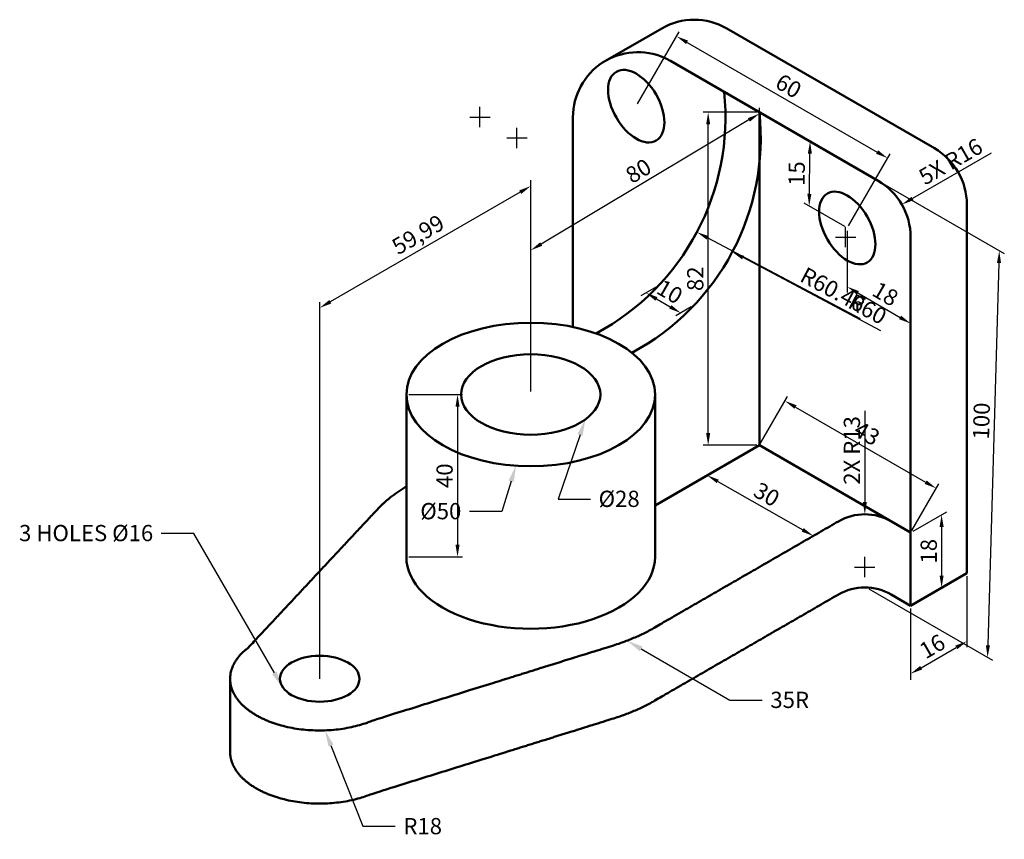
# Model space of a CAD drawing. Units: millimetres. Extents: x -6 to 237, y 25 to 227.
import ezdxf
from ezdxf import colors
from ezdxf.entities.mleader import LeaderData, LeaderLine
from ezdxf.math import Vec2, Vec3

# ---------------------------------------------------------------- set-up
doc = ezdxf.new("R2010")
doc.units = ezdxf.units.MM
doc.layers.add('M-DIMS', color=2, linetype='Continuous', lineweight=25)
doc.layers.add('M-OUTL', color=7, linetype='Continuous', lineweight=50)
doc.styles.get("Standard").update_dxf_attribs({"font": 'arial.ttf'})
doc.dimstyles.new('ISO-25', dxfattribs={"dimtxt": 4, "dimasz": 3, "dimexe": 1.25, "dimexo": 0.625, "dimtad": 1, "dimtxsty": 'Standard', "dimcen": 2.5, "dimadec": 0, "dimazin": 0, "dimtfac": 1, "dimtofl": 0, "dimtmove": 0, "dimatfit": 3, "dimfxl": 1, "dimarcsym": 0})

# ---------------------------------------------------------------- blocks, each defined once
blk = doc.blocks.new('*D1')
at = {"layer": 'Defpoints', "color": 0, "transparency": 16777216}
for p in [(227.4, 90.98), (213.54, 82.98), (227.4, 74.21)]:
    blk.add_point(p, dxfattribs=at)
at = {"layer": 'M-DIMS', "color": 0, "lineweight": -2, "transparency": 16777216}
for p, q in [((227.4, 90.26), (227.4, 72.76)), ((213.54, 82.26), (213.54, 64.76)), ((216.14, 67.71), (224.8, 72.71))]:
    blk.add_line(p, q, dxfattribs=at)
at = {"layer": 'M-DIMS', "color": 0, "transparency": 16777216}
for points in [[(224.55, 73.14), (225.05, 72.27), (227.4, 74.21)], [(215.89, 68.14), (216.39, 67.27), (213.54, 66.21)]]:
    blk.add_solid(points, dxfattribs=at)
at = {"layer": 'M-DIMS', "color": 0, "transparency": 16777216, "insert": (219.14, 72.52), "char_height": 4, "attachment_point": 5, "rotation": 30}
blk.add_mtext('16', dxfattribs=at)
blk = doc.blocks.new('*D2')
at = {"layer": 'Defpoints', "color": 0, "transparency": 16777216}
for p in [(145.99, 205.98), (207.88, 193.18), (197.95, 175.98)]:
    blk.add_point(p, dxfattribs=at)
at = {"layer": 'M-DIMS', "color": 0, "lineweight": -2, "transparency": 16777216}
for p, q in [((146.3, 206.52), (156.55, 224.26)), ((158.52, 221.68), (205.29, 194.68)), ((198.27, 176.52), (208.51, 194.26))]:
    blk.add_line(p, q, dxfattribs=at)
at = {"layer": 'M-DIMS', "color": 0, "transparency": 16777216}
for points in [[(158.77, 222.11), (158.27, 221.25), (155.92, 223.18)], [(205.54, 195.11), (205.04, 194.25), (207.88, 193.18)]]:
    blk.add_solid(points, dxfattribs=at)
at = {"layer": 'M-DIMS', "color": 0, "transparency": 16777216, "insert": (183.24, 210.49), "char_height": 4, "attachment_point": 5, "rotation": 330}
blk.add_mtext('60', dxfattribs=at)
blk = doc.blocks.new('*D3')
at = {"layer": 'Defpoints', "color": 0, "transparency": 16777216}
for p in [(188.78, 197.27), (198.15, 191.87), (197.95, 175.98)]:
    blk.add_point(p, dxfattribs=at)
at = {"layer": 'M-DIMS', "color": 0, "lineweight": -2, "transparency": 16777216}
for p, q in [((197.53, 192.22), (187.54, 197.99)), ((188.62, 184.39), (188.74, 194.27)), ((197.33, 176.34), (187.34, 182.1))]:
    blk.add_line(p, q, dxfattribs=at)
at = {"layer": 'M-DIMS', "color": 0, "transparency": 16777216}
for points in [[(188.24, 194.28), (189.24, 194.27), (188.78, 197.27)], [(188.12, 184.39), (189.12, 184.38), (188.58, 181.39)]]:
    blk.add_solid(points, dxfattribs=at)
at = {"layer": 'M-DIMS', "color": 0, "transparency": 16777216, "insert": (186.01, 189.36), "char_height": 4, "attachment_point": 5, "rotation": 89.2938}
blk.add_mtext('15', dxfattribs=at)
blk = doc.blocks.new('*D4')
at = {"layer": 'Defpoints', "color": 0, "transparency": 16777216}
for p in [(197.95, 175.98), (213.54, 166.92), (213.54, 152.46)]:
    blk.add_point(p, dxfattribs=at)
at = {"layer": 'M-DIMS', "color": 0, "lineweight": -2, "transparency": 16777216}
for p, q in [((197.95, 175.26), (197.95, 160.07)), ((213.54, 166.2), (213.54, 151.01)), ((200.55, 160.01), (210.95, 153.96))]:
    blk.add_line(p, q, dxfattribs=at)
at = {"layer": 'M-DIMS', "color": 0, "transparency": 16777216}
for points in [[(200.8, 160.44), (200.3, 159.57), (197.95, 161.51)], [(211.2, 154.4), (210.7, 153.53), (213.54, 152.46)]]:
    blk.add_solid(points, dxfattribs=at)
at = {"layer": 'M-DIMS', "color": 0, "transparency": 16777216, "insert": (207.09, 159.29), "char_height": 4, "attachment_point": 5, "rotation": 329.8439}
blk.add_mtext('18', dxfattribs=at)
blk = doc.blocks.new('*D5')
at = {"layer": 'Defpoints', "color": 0, "transparency": 16777216}
for p in [(163.47, 115.07), (189.58, 100.16), (189.58, 100.16)]:
    blk.add_point(p, dxfattribs=at)
at = {"layer": 'M-DIMS', "color": 0, "lineweight": -2, "transparency": 16777216}
for p, q in [((164.09, 115.43), (164.72, 115.79)), ((166.07, 113.58), (186.98, 101.64)), ((190.21, 100.52), (190.83, 100.88))]:
    blk.add_line(p, q, dxfattribs=at)
at = {"layer": 'M-DIMS', "color": 0, "transparency": 16777216}
for points in [[(166.32, 114.01), (165.82, 113.15), (163.47, 115.07)], [(187.22, 102.08), (186.73, 101.21), (189.58, 100.16)]]:
    blk.add_solid(points, dxfattribs=at)
at = {"layer": 'M-DIMS', "color": 0, "transparency": 16777216, "insert": (177.85, 109.93), "char_height": 4, "attachment_point": 5, "rotation": 330.2759}
blk.add_mtext('30', dxfattribs=at)
blk = doc.blocks.new('*D6')
at = {"layer": 'Defpoints', "color": 0, "transparency": 16777216}
for p in [(213.54, 100.98), (221.18, 87.39), (213.54, 82.98)]:
    blk.add_point(p, dxfattribs=at)
at = {"layer": 'M-DIMS', "color": 0, "lineweight": -2, "transparency": 16777216}
for p, q in [((214.17, 101.34), (222.43, 106.11)), ((221.18, 102.39), (221.18, 90.39)), ((214.17, 83.34), (222.43, 88.11))]:
    blk.add_line(p, q, dxfattribs=at)
at = {"layer": 'M-DIMS', "color": 0, "transparency": 16777216}
for points in [[(220.68, 102.39), (221.68, 102.39), (221.18, 105.39)], [(220.68, 90.39), (221.68, 90.39), (221.18, 87.39)]]:
    blk.add_solid(points, dxfattribs=at)
at = {"layer": 'M-DIMS', "color": 0, "transparency": 16777216, "insert": (218.52, 96.39), "char_height": 4, "attachment_point": 5, "rotation": 90}
blk.add_mtext('18', dxfattribs=at)
blk = doc.blocks.new('*D7')
at = {"layer": 'Defpoints', "color": 0, "transparency": 16777216}
for p in [(68.05, 156.31), (120.01, 134.98), (68.05, 105)]:
    blk.add_point(p, dxfattribs=at)
at = {"layer": 'M-DIMS', "color": 0, "lineweight": -2, "transparency": 16777216}
for p, q in [((120.01, 135.7), (120.01, 187.73)), ((117.41, 184.79), (70.65, 157.81)), ((68.05, 105.72), (68.05, 157.75))]:
    blk.add_line(p, q, dxfattribs=at)
at = {"layer": 'M-DIMS', "color": 0, "transparency": 16777216}
for points in [[(117.16, 185.22), (117.66, 184.35), (120.01, 186.29)], [(70.4, 158.24), (70.9, 157.38), (68.05, 156.31)]]:
    blk.add_solid(points, dxfattribs=at)
at = {"layer": 'M-DIMS', "color": 0, "transparency": 16777216, "insert": (92.52, 173.92), "char_height": 4, "attachment_point": 5, "rotation": 29.9808}
blk.add_mtext('59,99', dxfattribs=at)
blk = doc.blocks.new('*D8')
at = {"layer": 'Defpoints', "color": 0, "transparency": 16777216}
for p in [(176.3, 203.27), (120.01, 170.48), (120.01, 169.63)]:
    blk.add_point(p, dxfattribs=at)
at = {"layer": 'M-DIMS', "color": 0, "lineweight": -2, "transparency": 16777216}
for p, q in [((176.3, 203.99), (176.3, 205.58)), ((173.73, 202.59), (122.59, 172.02)), ((120.01, 170.35), (120.01, 171.94))]:
    blk.add_line(p, q, dxfattribs=at)
at = {"layer": 'M-DIMS', "color": 0, "transparency": 16777216}
for points in [[(173.47, 203.01), (173.98, 202.16), (176.3, 204.12)], [(122.33, 172.45), (122.84, 171.59), (120.01, 170.48)]]:
    blk.add_solid(points, dxfattribs=at)
at = {"layer": 'M-DIMS', "color": 0, "transparency": 16777216, "insert": (146.79, 189.59), "char_height": 4, "attachment_point": 5, "rotation": 30.8638}
blk.add_mtext('80', dxfattribs=at)
blk = doc.blocks.new('*D9')
at = {"layer": 'Defpoints', "color": 0, "transparency": 16777216}
for p in [(151.56, 161.87), (160.18, 156.89), (156.97, 155.05)]:
    blk.add_point(p, dxfattribs=at)
at = {"layer": 'M-DIMS', "color": 0, "lineweight": -2, "transparency": 16777216}
for p, q in [((150.94, 161.5), (147.11, 159.3)), ((150.96, 158.52), (154.38, 156.55)), ((159.55, 156.53), (155.72, 154.32))]:
    blk.add_line(p, q, dxfattribs=at)
at = {"layer": 'M-DIMS', "color": 0, "transparency": 16777216}
for points in [[(151.21, 158.95), (150.71, 158.08), (148.36, 160.02)], [(154.63, 156.98), (154.13, 156.11), (156.97, 155.05)]]:
    blk.add_solid(points, dxfattribs=at)
at = {"layer": 'M-DIMS', "color": 0, "transparency": 16777216, "insert": (154, 159.84), "char_height": 4, "attachment_point": 5, "rotation": 330}
blk.add_mtext('10', dxfattribs=at)
blk = doc.blocks.new('*D10')
at = {"layer": 'Defpoints', "color": 0, "transparency": 16777216}
for p in [(205.54, 187.6), (202.65, 87.47), (232.49, 70.24)]:
    blk.add_point(p, dxfattribs=at)
at = {"layer": 'M-DIMS', "color": 0, "lineweight": -2, "transparency": 16777216}
for p, q in [((206.16, 187.24), (236.61, 169.66)), ((235.3, 167.37), (232.58, 73.24)), ((203.26, 87.11), (233.72, 69.53))]:
    blk.add_line(p, q, dxfattribs=at)
at = {"layer": 'M-DIMS', "color": 0, "transparency": 16777216}
for points in [[(234.8, 167.38), (235.8, 167.35), (235.38, 170.37)], [(232.08, 73.25), (233.08, 73.22), (232.49, 70.24)]]:
    blk.add_solid(points, dxfattribs=at)
at = {"layer": 'M-DIMS', "color": 0, "transparency": 16777216, "insert": (231.5, 128.44), "char_height": 4, "attachment_point": 5, "rotation": 88.345}
blk.add_mtext('100', dxfattribs=at)
blk = doc.blocks.new('*D11')
at = {"layer": 'Defpoints', "color": 0, "transparency": 16777216}
for p in [(89.39, 134.98), (89.39, 94.98), (101.99, 94.98)]:
    blk.add_point(p, dxfattribs=at)
at = {"layer": 'M-DIMS', "color": 0, "lineweight": -2, "transparency": 16777216}
for p, q in [((90.02, 134.98), (103.24, 134.98)), ((101.99, 131.98), (101.99, 97.98)), ((90.02, 94.98), (103.24, 94.98))]:
    blk.add_line(p, q, dxfattribs=at)
at = {"layer": 'M-DIMS', "color": 0, "transparency": 16777216}
for points in [[(101.49, 131.98), (102.49, 131.98), (101.99, 134.98)], [(101.49, 97.98), (102.49, 97.98), (101.99, 94.98)]]:
    blk.add_solid(points, dxfattribs=at)
at = {"layer": 'M-DIMS', "color": 0, "transparency": 16777216, "insert": (99.32, 114.98), "char_height": 4, "attachment_point": 5, "rotation": 90}
blk.add_mtext('40', dxfattribs=at)
blk = doc.blocks.new('*D12')
at = {"layer": 'Defpoints', "color": 0, "transparency": 16777216}
for p in [(176.3, 122.48), (219.84, 111.89), (213.54, 100.98)]:
    blk.add_point(p, dxfattribs=at)
at = {"layer": 'M-DIMS', "color": 0, "lineweight": -2, "transparency": 16777216}
for p, q in [((176.61, 123.02), (183.23, 134.47)), ((185.2, 131.89), (217.24, 113.39)), ((213.85, 101.52), (220.47, 112.97))]:
    blk.add_line(p, q, dxfattribs=at)
at = {"layer": 'M-DIMS', "color": 0, "transparency": 16777216}
for points in [[(185.45, 132.32), (184.95, 131.46), (182.6, 133.39)], [(217.49, 113.82), (216.99, 112.96), (219.84, 111.89)]]:
    blk.add_solid(points, dxfattribs=at)
at = {"layer": 'M-DIMS', "color": 0, "transparency": 16777216, "insert": (202.56, 124.95), "char_height": 4, "attachment_point": 5, "rotation": 330}
blk.add_mtext('43', dxfattribs=at)
blk = doc.blocks.new('*D13')
at = {"layer": 'Defpoints', "color": 0, "transparency": 16777216}
for p in [(163.7, 204.48), (176.3, 204.48), (176.3, 122.48)]:
    blk.add_point(p, dxfattribs=at)
at = {"layer": 'M-DIMS', "color": 0, "lineweight": -2, "transparency": 16777216}
for p, q in [((175.68, 204.48), (162.45, 204.48)), ((163.7, 125.48), (163.7, 201.48)), ((175.68, 122.48), (162.45, 122.48))]:
    blk.add_line(p, q, dxfattribs=at)
at = {"layer": 'M-DIMS', "color": 0, "transparency": 16777216}
for points in [[(163.2, 201.48), (164.2, 201.48), (163.7, 204.48)], [(163.2, 125.48), (164.2, 125.48), (163.7, 122.48)]]:
    blk.add_solid(points, dxfattribs=at)
at = {"layer": 'M-DIMS', "color": 0, "transparency": 16777216, "insert": (161.04, 163.48), "char_height": 4, "attachment_point": 5, "rotation": 90}
blk.add_mtext('82', dxfattribs=at)
blk = doc.blocks.new('*D14')
at = {"layer": 'Defpoints', "color": 0, "transparency": 16777216}
for p in [(116.63, 198.17), (169.65, 170.08)]:
    blk.add_point(p, dxfattribs=at)
at = {"layer": 'M-DIMS', "color": 0, "lineweight": -2, "transparency": 16777216}
for p, q in [((116.63, 195.67), (116.63, 200.67)), ((114.13, 198.17), (119.13, 198.17)), ((206.23, 150.69), (172.3, 168.67))]:
    blk.add_line(p, q, dxfattribs=at)
at = {"layer": 'M-DIMS', "color": 0, "transparency": 16777216}
blk.add_solid([(172.53, 169.11), (172.07, 168.23), (169.65, 170.08)], dxfattribs=at)
at = {"layer": 'M-DIMS', "color": 0, "transparency": 16777216, "insert": (202.71, 155.58), "char_height": 4, "attachment_point": 5, "rotation": 332.0773}
blk.add_mtext('R60', dxfattribs=at)
blk = doc.blocks.new('*D15')
at = {"layer": 'Defpoints', "color": 0, "transparency": 16777216}
for p in [(107.5, 203.27), (160.92, 174.95)]:
    blk.add_point(p, dxfattribs=at)
at = {"layer": 'M-DIMS', "color": 0, "lineweight": -2, "transparency": 16777216}
for p, q in [((107.5, 200.77), (107.5, 205.77)), ((105, 203.27), (110, 203.27)), ((201.18, 153.62), (163.57, 173.55))]:
    blk.add_line(p, q, dxfattribs=at)
at = {"layer": 'M-DIMS', "color": 0, "transparency": 16777216}
blk.add_solid([(163.81, 173.99), (163.34, 173.11), (160.92, 174.95)], dxfattribs=at)
at = {"layer": 'M-DIMS', "color": 0, "transparency": 16777216, "insert": (194.23, 160.32), "char_height": 4, "attachment_point": 5, "rotation": 332.0776}
blk.add_mtext('R60.46', dxfattribs=at)
blk = doc.blocks.new('*D16')
at = {"layer": 'Defpoints', "color": 0, "transparency": 16777216}
for p in [(211.4, 181.74), (197.54, 173.74)]:
    blk.add_point(p, dxfattribs=at)
at = {"layer": 'M-DIMS', "color": 0, "lineweight": -2, "transparency": 16777216}
for p, q in [((233.4, 194.44), (214, 183.24)), ((197.54, 171.24), (197.54, 176.24)), ((195.04, 173.74), (200.04, 173.74))]:
    blk.add_line(p, q, dxfattribs=at)
at = {"layer": 'M-DIMS', "color": 0, "transparency": 16777216}
blk.add_solid([(213.75, 183.67), (214.25, 182.81), (211.4, 181.74)], dxfattribs=at)
at = {"layer": 'M-DIMS', "color": 0, "transparency": 16777216, "insert": (223.66, 191.9), "char_height": 4, "attachment_point": 5, "rotation": 29.9982}
blk.add_mtext('5X R16', dxfattribs=at)
blk = doc.blocks.new('*D17')
at = {"layer": 'Defpoints', "color": 0, "transparency": 16777216}
for p in [(202.27, 105.47), (202.27, 92.47)]:
    blk.add_point(p, dxfattribs=at)
at = {"layer": 'M-DIMS', "color": 0, "lineweight": -2, "transparency": 16777216}
for p, q in [((202.27, 130.94), (202.27, 108.47)), ((202.27, 89.97), (202.27, 94.97)), ((199.77, 92.47), (204.77, 92.47))]:
    blk.add_line(p, q, dxfattribs=at)
at = {"layer": 'M-DIMS', "color": 0, "transparency": 16777216}
blk.add_solid([(201.77, 108.47), (202.77, 108.47), (202.27, 105.47)], dxfattribs=at)
at = {"layer": 'M-DIMS', "color": 0, "transparency": 16777216, "insert": (199.6, 121.21), "char_height": 4, "attachment_point": 5, "rotation": 89.9994}
blk.add_mtext('2X R13', dxfattribs=at)

msp = doc.modelspace()

# ---------------------------------------------------------------- linework, layer by layer
at = {"layer": 'M-DIMS'}
msp.add_line((68.049, 64.978), (68.049, 107.557), dxfattribs=at)
at = {"layer": 'M-OUTL'}
for p, q in [((138.403, 217.122), (152.259, 225.122)), ((219.398, 195.597), (168.259, 225.122)), ((205.541, 187.597), (154.403, 217.122)), ((205.541, 187.597), (154.403, 217.122)), ((176.302, 204.478), (176.302, 122.478)), ((130.403, 203.265), (130.403, 151.606)), ((227.398, 90.978), (227.398, 181.74)), ((213.541, 82.978), (213.541, 173.74)), ((89.392, 134.978), (89.392, 94.978)), ((150.629, 134.978), (150.629, 94.978)), ((176.302, 122.478), (150.629, 107.656)), ((213.541, 100.978), (176.302, 122.478)), ((213.541, 82.978), (213.541, 100.978)), ((213.541, 82.978), (227.398, 90.978)), ((208.773, 85.731), (213.541, 82.978)), ((46.004, 46.922), (46.004, 64.978))]:
    msp.add_line(p, q, dxfattribs=at)
for centre, radius, start, end in [((160.259, 211.265), 16, 60, 120), ((146.403, 203.265), 16, 65.96309, 180), ((146.403, 203.265), 16, 60, 65.96309), ((107.498, 203.267), 60.464, 298.25907, 5.89628), ((116.634, 198.175), 60, 298.12497, 6.03038), ((211.398, 181.74), 16, 0, 60), ((197.541, 173.74), 16, 0, 60), ((202.273, 92.473), 13, 60, 120), ((202.273, 74.473), 13, 60, 120)]:
    msp.add_arc(centre, radius, start, end, dxfattribs=at)
for centre, major_axis in [((145.991, 205.978), (4.899, -8.485)), ((197.953, 175.978), (4.899, -8.485)), ((120.011, 134.978), (-30.619, 0)), ((120.011, 134.978), (-17.146, 0)), ((68.049, 64.978), (-9.798, 0))]:
    msp.add_ellipse(centre, major_axis=major_axis, ratio=0.5773503, dxfattribs=at)
msp.add_ellipse((120.011, 94.978), major_axis=(-30.619, 0), ratio=0.5773503, start_param=0, end_param=3.1415927, dxfattribs=at)
for points, weights, knots in [([(89.392, 112.299), (84.799, 109.592), (81.819, 106.216), (66.16, 89.449), (50.501, 72.682), (39.014, 63.961), (52.243, 56.105), (65.472, 48.25), (80.895, 54.634), (110.426, 63.853), (139.957, 73.072), (146.223, 74.974), (151.097, 77.938), (173.435, 90.834), (195.773, 103.731)], [0.996613645118, 0.986806868253, 1, 1, 1, 0.757877776403, 1, 0.757877776403, 1, 1, 1, 0.98663647273, 1, 1, 1], [1.0447145, 1.0447145, 1.0447145, 1.3484128, 1.3484128, 2.3484128, 2.3484128, 3.7698975, 3.7698975, 5.1913822, 5.1913822, 6.1913822, 6.1913822, 6.5187157, 6.5187157, 7.3917018, 7.3917018, 7.3917018]), ([(46.004, 46.922), (46.043, 41.787), (52.243, 38.105), (65.472, 30.25), (80.895, 36.634), (110.426, 45.853), (139.957, 55.072), (146.223, 56.974), (151.097, 59.938), (173.435, 72.834), (195.773, 85.731)], [0.879633594104, 0.86976818109, 1, 0.757877776403, 1, 1, 1, 0.98663647273, 1, 1, 1], [3.0053145, 3.0053145, 3.0053145, 3.7698975, 3.7698975, 5.1913822, 5.1913822, 6.1913822, 6.1913822, 6.5187157, 6.5187157, 7.3917018, 7.3917018, 7.3917018])]:
    msp.add_rational_spline(points, weights, degree=2, knots=knots, dxfattribs=at)

# ---------------------------------------------------------------- dimensions: what is measured, and where the dimension line sits
at = {"layer": 'M-DIMS'}
for p1, p2, distance, picture, middle in [((145.991, 205.978), (197.953, 175.978), 19.862, '*D2', (183.237, 210.489)), ((120.011, 134.978), (68.049, 105.001), -44.443, '*D7', (92.516, 173.921)), ((213.541, 100.978), (213.541, 82.978), 7.642, '*D6', (218.516, 96.39)), ((213.541, 82.978), (227.398, 90.978), -14.523, '*D1', (219.136, 72.518))]:
    dim = msp.add_aligned_dim(p1=p1, p2=p2, distance=distance, dimstyle='ISO-25', override={"dimclrd": 0, "dimclre": 0, "dimclrt": 0}, dxfattribs=at)
    dim.commit()
    dim.dimension.update_dxf_attribs({"geometry": picture, "text_midpoint": middle})
for center, mpoint, override, picture, middle in [((107.498, 203.267), (160.923, 174.953), {"dimdec": 2, "dimlfac": 1, "dimrnd": 0, "dimzin": 0, "dimdsep": 46, "dimlunit": 2}, '*D15', (192.978, 157.965)), ((116.634, 198.175), (169.649, 170.078), {"dimdec": 0, "dimlfac": 1, "dimrnd": 0, "dimzin": 0, "dimdsep": 46, "dimlunit": 2}, '*D14', (201.458, 153.22))]:
    dim = msp.add_radius_dim(center=center, mpoint=mpoint, dimstyle='ISO-25', override=override, dxfattribs=at)
    dim.commit()
    dim.dimension.update_dxf_attribs({"geometry": picture, "text_midpoint": middle, "dimtype": 164})
for p1, p2, distance, text, picture, middle in [((176.302, 203.267), (120.011, 169.625), -0.736, '80', '*D8', (146.788, 189.593)), ((197.953, 175.978), (198.149, 191.865), 9.435, '15', '*D3', (186.015, 189.364)), ((197.953, 175.978), (213.541, 166.921), -12.507, '18', '*D4', (207.087, 159.291)), ((151.564, 161.866), (160.176, 156.894), -3.202, '10', '*D9', (154.002, 159.841)), ((163.466, 115.067), (189.581, 100.156), 0, '30', '*D5', (177.847, 109.929))]:
    dim = msp.add_aligned_dim(p1=p1, p2=p2, distance=distance, text=text, dimstyle='ISO-25', override={"dimclrd": 0, "dimclre": 0, "dimclrt": 0}, dxfattribs=at)
    dim.commit()
    dim.dimension.update_dxf_attribs({"geometry": picture, "text_midpoint": middle})
for base, p1, p2, angle, picture, middle in [((163.702, 204.478), (176.302, 122.478), (176.302, 204.478), 90, '*D13', (161.035, 163.478)), ((101.992, 94.978), (89.392, 134.978), (89.392, 94.978), 270, '*D11', (99.325, 114.978)), ((219.841, 111.89), (176.302, 122.478), (213.541, 100.978), 330, '*D12', (202.556, 124.951))]:
    dim = msp.add_linear_dim(base=base, p1=p1, p2=p2, angle=angle, dimstyle='ISO-25', override={"dimdec": 0, "dimlfac": 1, "dimrnd": 0, "dimzin": 0, "dimdsep": 46, "dimlunit": 2}, dxfattribs=at)
    dim.commit()
    dim.dimension.update_dxf_attribs({"geometry": picture, "text_midpoint": middle})
for center, mpoint, text, picture, middle in [((197.541, 173.74), (211.398, 181.74), '5X <>', '*D16', (223.661, 191.9)), ((202.273, 92.473), (202.273, 105.473), '2X <>', '*D17', (199.605, 121.208))]:
    dim = msp.add_radius_dim(center=center, mpoint=mpoint, text=text, dimstyle='ISO-25', override={"dimdec": 0, "dimlfac": 1, "dimrnd": 0, "dimzin": 0, "dimdsep": 46, "dimlunit": 2}, dxfattribs=at)
    dim.commit()
    dim.dimension.update_dxf_attribs({"geometry": picture, "text_midpoint": middle})
dim = msp.add_linear_dim(base=(232.491, 70.238), p1=(205.541, 187.597), p2=(202.648, 87.467), angle=268.345, text='100', dimstyle='ISO-25', override={"dimclrd": 0, "dimclre": 0, "dimclrt": 0}, dxfattribs=at)
dim.commit()
dim.dimension.update_dxf_attribs({"geometry": '*D10', "text_midpoint": (234.17, 128.359), "dimtype": 161})

# ---------------------------------------------------------------- leaders
ml = msp.add_multileader_mtext('Standard', dxfattribs=at)
ml.set_content('%%C28', color=256)
ml.set_leader_properties()
ml.build(insert=Vec2(0, 0))
ctx = ml.context
ctx.base_point, ctx.plane_origin = Vec3(134.731, 109.208), Vec3(133.453, 128.832)
notes = []
notes.append((ctx, [(0, (1, 1, 0), (126.731, 109.208), (1, 0), 8, [(0, [(133.453, 128.832)], 0, [])])]))
ctx.mtext.insert, ctx.mtext.flow_direction = Vec3(136.731, 111.288), 5
ml = msp.add_multileader_mtext('Standard', dxfattribs=at)
ml.set_content('%%C50', color=256)
ml.set_leader_properties()
ml.build(insert=Vec2(0, 0))
ctx = ml.context
ctx.base_point, ctx.plane_origin = Vec3(90.862, 106.173), Vec3(130.208, 118.31)
ctx.text_align_type = 2
notes.append((ctx, [(0, (1, 1, 0), (112.931, 106.173), (-1, 0), 8, [(0, [(116.374, 117.426)], 0, [])])]))
ctx.mtext.insert, ctx.mtext.alignment, ctx.mtext.flow_direction = Vec3(102.931, 108.254), 3, 5
ml = msp.add_multileader_mtext('Standard', dxfattribs=at)
ml.set_content('3 HOLES %%C16', color=256)
ml.set_leader_properties()
ml.build(insert=Vec2(0, 0))
ctx = ml.context
ctx.base_point, ctx.plane_origin = Vec3(-10.166, 100.781), Vec3(58.906, 62.944)
ctx.text_align_type = 2
notes.append((ctx, [(0, (1, 1, 0), (37.061, 100.781), (-1, 0), 8, [(0, [(58.906, 62.944)], 0, [])])]))
ctx.mtext.insert, ctx.mtext.alignment, ctx.mtext.flow_direction = Vec3(27.061, 102.861), 3, 5
ml = msp.add_multileader_mtext('Standard', dxfattribs=at)
ml.set_content('35R', color=256)
ml.set_leader_properties()
ml.build(insert=Vec2(0, 0))
ctx = ml.context
ctx.base_point, ctx.plane_origin = Vec3(177.012, 59.754), Vec3(143.717, 74.358)
notes.append((ctx, [(0, (1, 1, 0), (169.012, 59.754), (1, 0), 8, [(0, [(143.717, 74.358)], 0, [])])]))
ctx.mtext.insert, ctx.mtext.flow_direction = Vec3(179.012, 61.79), 5
ml = msp.add_multileader_mtext('Standard', dxfattribs=at)
ml.set_content('R18', color=256)
ml.set_leader_properties()
ml.build(insert=Vec2(0, 0))
ctx = ml.context
ctx.base_point, ctx.plane_origin = Vec3(86.647, 28.669), Vec3(69.363, 52.273)
notes.append((ctx, [(1, (1, 1, 0), (78.647, 28.669), (1, 0), 8, [(0, [(69.363, 52.273)], 0, [])])]))
ctx.mtext.insert, ctx.mtext.flow_direction = Vec3(88.647, 30.703), 5
for ctx, leaders in notes:
    for number, flags, end, landing, length, lines in leaders:
        leader = LeaderData()
        leader.index, (leader.has_last_leader_line, leader.has_dogleg_vector, leader.attachment_direction) = number, flags
        leader.last_leader_point, leader.dogleg_vector, leader.dogleg_length = Vec3(end), Vec3(landing), length
        for number, points, colour, breaks in lines:
            line = LeaderLine()
            line.index, line.vertices, line.color, line.breaks = number, Vec3.list(points), colors.encode_raw_color(colour), breaks
            leader.lines.append(line)
        ctx.leaders.append(leader)

doc.saveas('drawing.dxf')
